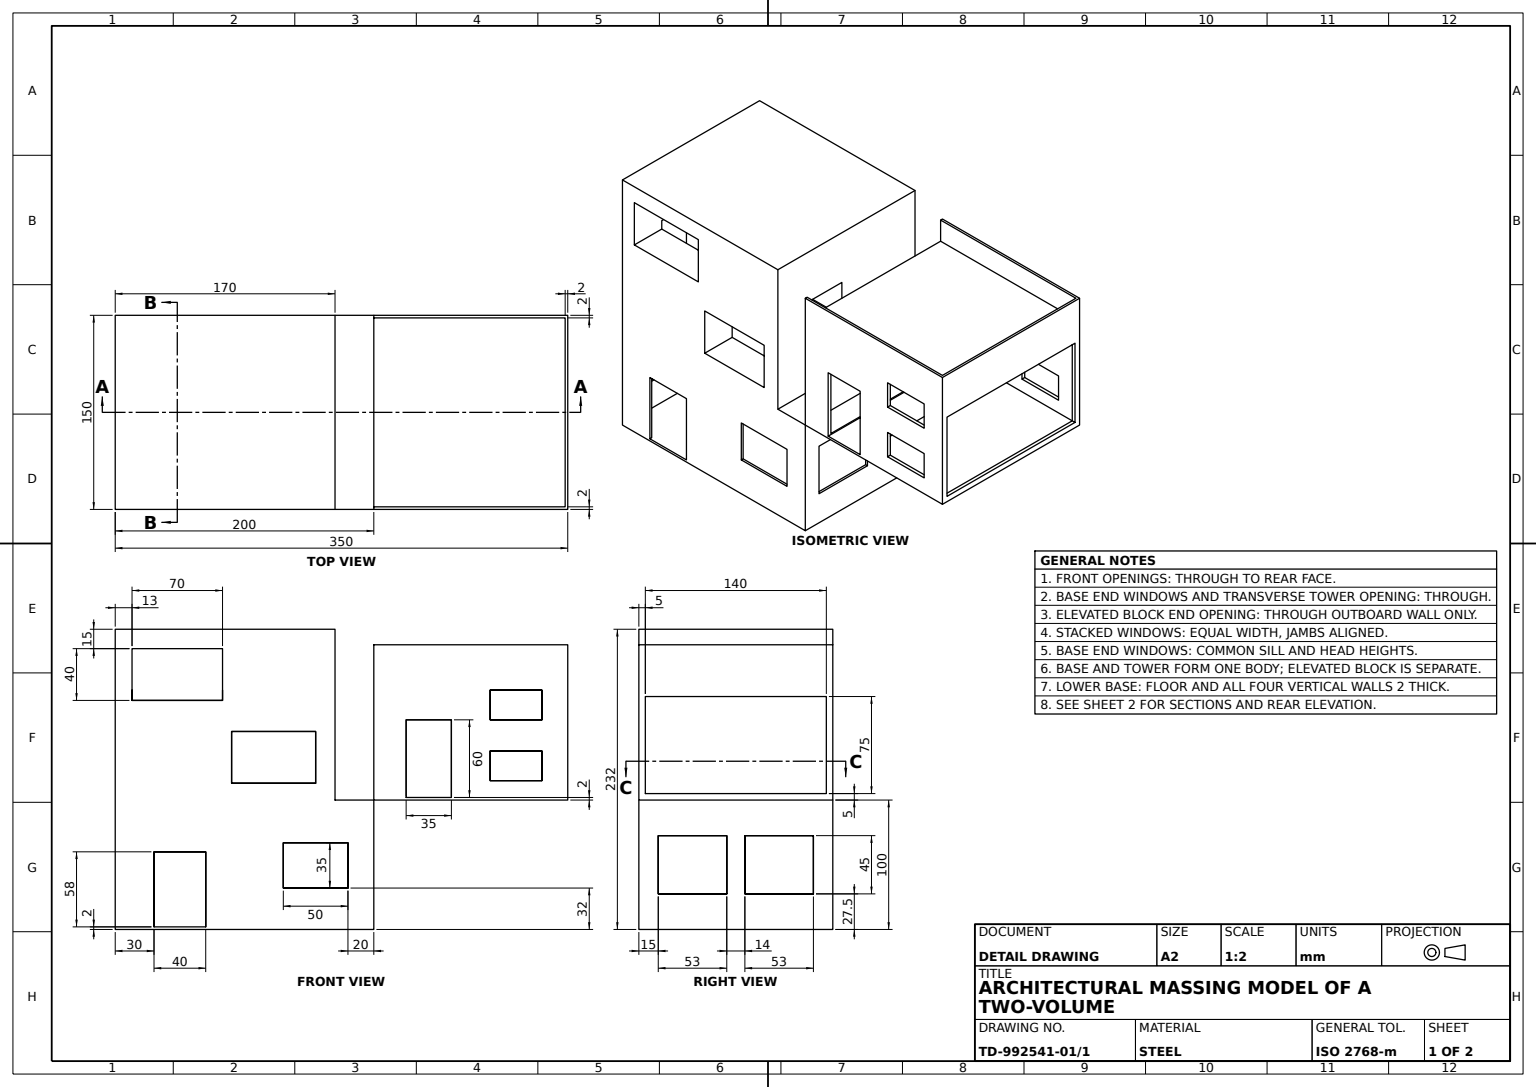
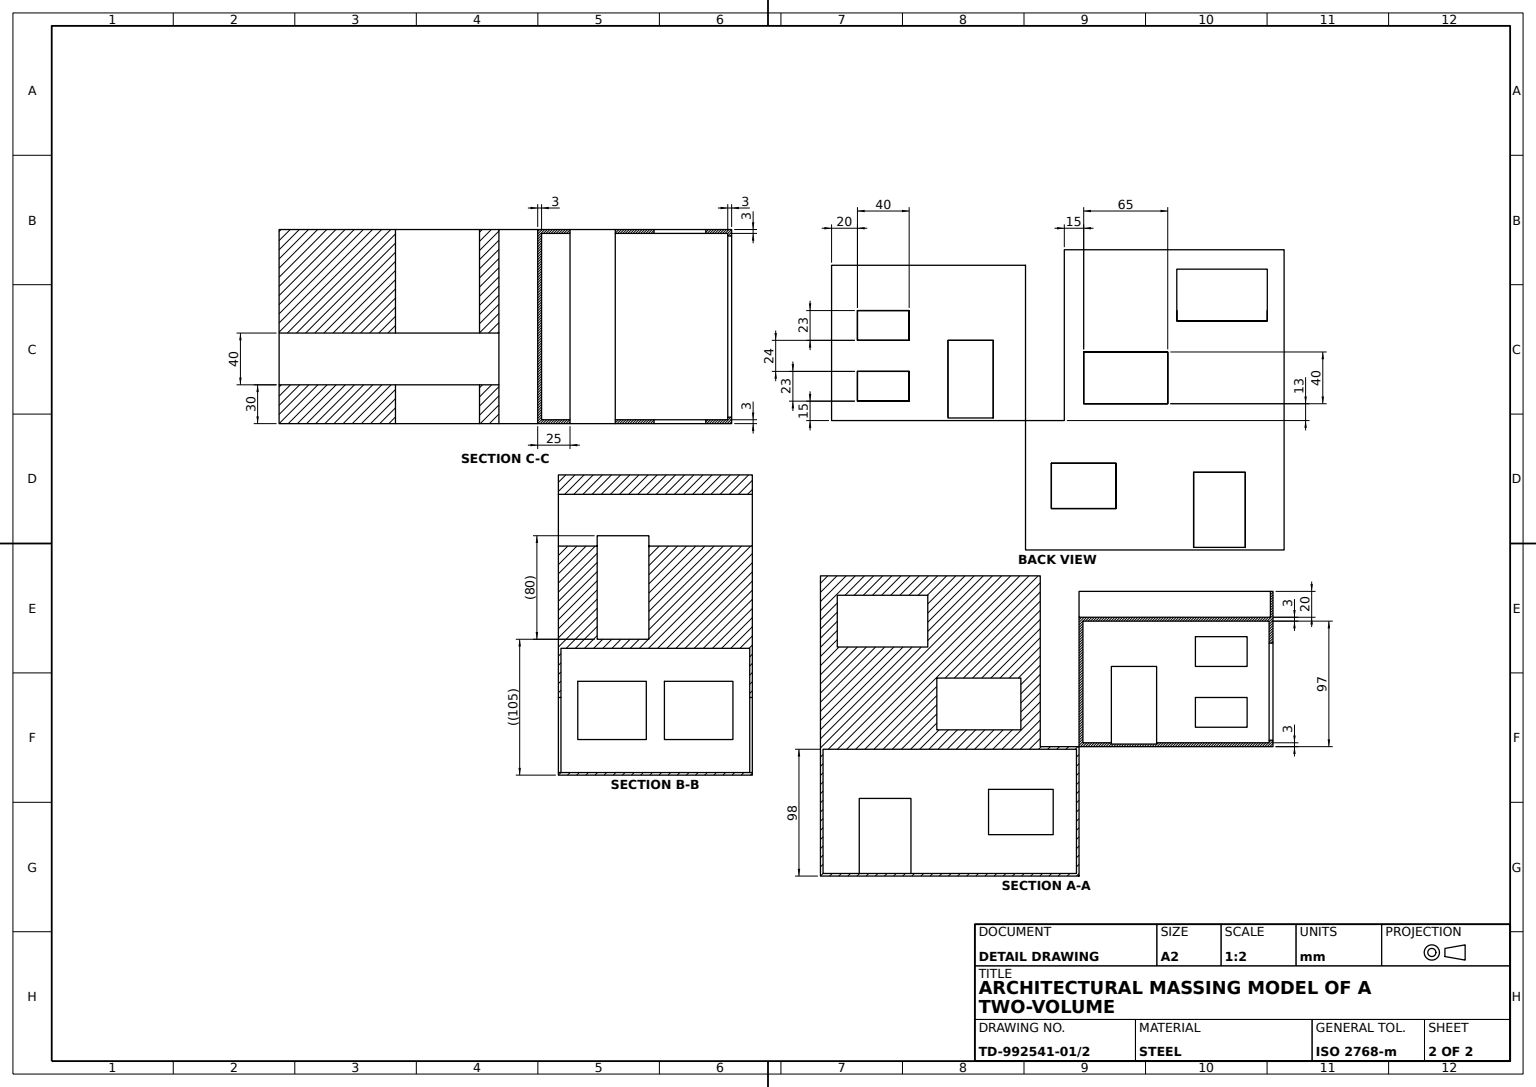
SolidWorks part; units mm, degrees
material "Plain Carbon Steel"
ref_plane "Front Plane" through (0, 0, 0) normal (0, 0, 1) x (1, 0, 0)
ref_plane "Top Plane" through (0, 0, 0) normal (0, 1, 0) x (1, 0, 0)
ref_plane "Right Plane" through (0, 0, 0) normal (1, 0, 0) x (0, 0, -1)
sketch "Base Block Sketch" plane through (0, 0, 0) normal (0, 1, 0) x (1, 0, 0)
  line L1 (0, 0) -> (200, 0)
  line L2 (0, 0) -> (0, 150)
  line L3 (0, 150) -> (200, 150)
  line L4 (200, 0) -> (200, 150)
  dimension "D1" = 200
  dimension "D2" = 150
extrude "Base Block" add sketch "Base Block Sketch" along normal blind 100
sketch "Base Door Opening Sketch" plane through (0, 0, 0) normal (0, 0, 1) x (1, 0, 0)
  line L1 (30, 2) -> (70, 2)
  line L2 (30, 2) -> (30, 60)
  line L3 (30, 60) -> (70, 60)
  line L4 (70, 2) -> (70, 60)
  dimension "D1" = 2
  dimension "D2" = 30
  dimension "D3" = 40
  dimension "D4" = 58
extrude "Base Door Opening" cut sketch "Base Door Opening Sketch" against normal blind 270
sketch "Base Hollow Sketch" plane through (0, 100, 0) normal (0, 1, 0) x (1, 0, 0)
  line L0 (200, 0) -> (200, 150) construction
  line L1 (2, 148) -> (198, 148)
  line L2 (2, 148) -> (2, 2)
  line L3 (2, 2) -> (198, 2)
  line L4 (198, 148) -> (198, 2)
  line L5 (200, 150) -> (0, 150) construction
  line L6 (0, 150) -> (0, 0) construction
  line L7 (0, 0) -> (200, 0) construction
  dimension "D1" = 2
  dimension "D2" = 2
  dimension "D3" = 2
  dimension "D4" = 2
extrude "Base Hollow 2mm Wall" cut sketch "Base Hollow Sketch" against normal blind 98
sketch "Base Floor Slab Sketch" plane through (0, 100, 0) normal (0, 1, 0) x (1, 0, 0)
  line L1 (0, 150) -> (200, 150)
  line L2 (0, 150) -> (0, 0)
  line L3 (0, 0) -> (200, 0)
  line L4 (200, 150) -> (200, 0)
extrude "Base Floor Slab" add sketch "Base Floor Slab Sketch" against normal blind 2
sketch "Base Window Sketch" plane through (0, 0, 0) normal (0, 0, 1) x (1, 0, 0)
  line L1 (130, 32) -> (180, 32)
  line L2 (130, 32) -> (130, 67)
  line L3 (130, 67) -> (180, 67)
  line L4 (180, 32) -> (180, 67)
  dimension "D1" = 32
  dimension "D2" = 35
  dimension "D3" = 50
  dimension "D4" = 20
extrude "Base Window" cut sketch "Base Window Sketch" against normal blind 332
sketch "Base Side Windows Sketch" plane through (200, 0, 0) normal (1, 0, 0) x (0, 0, -1)
  line L0 (0, 0) -> (150, 0) construction
  line L1 (15, 27.5) -> (68, 27.5)
  line L2 (15, 27.5) -> (15, 72.5)
  line L3 (15, 72.5) -> (68, 72.5)
  line L4 (68, 27.5) -> (68, 72.5)
  line L5 (82, 27.5) -> (135, 27.5)
  line L6 (82, 27.5) -> (82, 72.5)
  line L7 (82, 72.5) -> (135, 72.5)
  line L8 (135, 27.5) -> (135, 72.5)
  dimension "D1" = 15
  dimension "D2" = 15
  dimension "D3" = 53
  dimension "D4" = 53
  dimension "D5" = 45
  dimension "D6" = 45
  dimension "D7" = 27.5
  dimension "D8" = 27.5
extrude "Base Side Windows" cut sketch "Base Side Windows Sketch" against normal blind 332
sketch "Side Block Sketch" plane through (0, 100, 0) normal (0, 1, 0) x (1, 0, 0)
  line L1 (200, 0) -> (350, 0)
  line L2 (200, 0) -> (200, 150)
  line L3 (200, 150) -> (350, 150)
  line L4 (350, 0) -> (350, 150)
  dimension "D1" = 150
  dimension "D2" = 150
extrude "Side Block" add sketch "Side Block Sketch" along normal blind 100 separate body
sketch "Side Block Hollow Sketch" plane through (0, 200, 0) normal (0, 1, 0) x (1, 0, 0)
  line L0 (200, 0) -> (350, 0) construction
  line L1 (203, 147) -> (347, 147)
  line L2 (203, 147) -> (203, 3)
  line L3 (203, 3) -> (347, 3)
  line L4 (347, 147) -> (347, 3)
  line L5 (350, 0) -> (350, 150) construction
  line L6 (350, 150) -> (200, 150) construction
  line L7 (200, 150) -> (200, 0) construction
  dimension "D1" = 3
  dimension "D2" = 3
  dimension "D3" = 3
  dimension "D4" = 3
extrude "Side Block Hollow 3mm Wall" cut sketch "Side Block Hollow Sketch" against normal blind 97
sketch "Side Block Floor Slab Sketch" plane through (0, 200, 0) normal (0, 1, 0) x (1, 0, 0)
  line L1 (200, 150) -> (350, 150)
  line L2 (200, 150) -> (200, 0)
  line L3 (200, 0) -> (350, 0)
  line L4 (350, 150) -> (350, 0)
extrude "Side Block Floor Slab" add sketch "Side Block Floor Slab Sketch" against normal blind 3
sketch "Side Block Door Sketch" plane through (0, 0, 0) normal (0, 0, 1) x (1, 0, 0)
  line L1 (225, 102) -> (260, 102)
  line L2 (225, 102) -> (225, 162)
  line L3 (225, 162) -> (260, 162)
  line L4 (260, 102) -> (260, 162)
  dimension "D1" = 2
  dimension "D2" = 25
  dimension "D3" = 35
  dimension "D4" = 60
extrude "Side Block Door Opening" cut sketch "Side Block Door Sketch" against normal blind 213
sketch "Side Block Windows Sketch" plane through (0, 0, 0) normal (0, 0, 1) x (1, 0, 0)
  line L1 (290, 115) -> (330, 115)
  line L2 (290, 115) -> (290, 138)
  line L3 (290, 138) -> (330, 138)
  line L4 (330, 115) -> (330, 138)
  line L5 (290, 162) -> (330, 162)
  line L6 (290, 162) -> (290, 185)
  line L7 (290, 185) -> (330, 185)
  line L8 (330, 162) -> (330, 185)
  dimension "D1" = 15
  dimension "D2" = 15
  dimension "D3" = 23
  dimension "D4" = 23
  dimension "D5" = 40
  dimension "D6" = 40
  dimension "D7" = 20
  dimension "D8" = 20
extrude "Side Block Windows" cut sketch "Side Block Windows Sketch" against normal blind 213
sketch "Side Block Front Opening Sketch" plane through (350, 0, 0) normal (1, 0, 0) x (0, 0, -1)
  line L0 (150, 200) -> (150, 100) construction
  line L1 (5, 105) -> (145, 105)
  line L2 (5, 105) -> (5, 180)
  line L3 (5, 180) -> (145, 180)
  line L4 (145, 105) -> (145, 180)
  dimension "D1" = 5
  dimension "D2" = 75
  dimension "D3" = 5
  dimension "D4" = 140
extrude "Side Block Front Opening" cut sketch "Side Block Front Opening Sketch" against normal blind 113
sketch "Parapet Front Sketch" plane through (0, 0, 0) normal (0, 0, 1) x (1, 0, 0)
  line L1 (200, 200) -> (350, 200)
  line L2 (200, 200) -> (200, 220)
  line L3 (200, 220) -> (350, 220)
  line L4 (350, 200) -> (350, 220)
  dimension "D1" = 20
  dimension "D2" = 150
extrude "Parapet Front" add sketch "Parapet Front Sketch" against normal blind 2
sketch "Parapet Side Sketch" plane through (350, 0, 0) normal (1, 0, 0) x (0, 0, -1)
  line L1 (2, 200) -> (149, 200)
  line L2 (2, 200) -> (2, 220)
  line L3 (2, 220) -> (149, 220)
  line L4 (149, 200) -> (149, 220)
  dimension "D1" = 20
  dimension "D2" = 147
extrude "Parapet Side" add sketch "Parapet Side Sketch" against normal blind 2
sketch "Parapet Back Sketch" plane through (0, 0, -150) normal (0, 0, -1) x (-1, 0, 0)
  line L1 (-350, 220) -> (-200, 220)
  line L2 (-350, 220) -> (-350, 200)
  line L3 (-350, 200) -> (-200, 200)
  line L4 (-200, 220) -> (-200, 200)
extrude "Parapet Back" add sketch "Parapet Back Sketch" against normal blind 2
sketch "Tower Sketch" plane through (0, 100, 0) normal (0, 1, 0) x (1, 0, 0)
  line L0 (0, 0) -> (200, 0) construction
  line L1 (0, 150) -> (170, 150)
  line L2 (0, 150) -> (0, 0)
  line L3 (0, 0) -> (170, 0)
  line L4 (170, 150) -> (170, 0)
  dimension "D1" = 170
extrude "Tower Extension" add sketch "Tower Sketch" along normal blind 132
sketch "Tower Windows Sketch" plane through (0, 0, 0) normal (0, 0, 1) x (1, 0, 0)
  line L0 (0, 232) -> (0, 0) construction
  line L1 (155, 113) -> (90, 113)
  line L2 (155, 113) -> (155, 153)
  line L3 (155, 153) -> (90, 153)
  line L4 (90, 113) -> (90, 153)
  line L5 (13, 217) -> (83, 217)
  line L6 (13, 217) -> (13, 177)
  line L7 (13, 177) -> (83, 177)
  line L8 (83, 217) -> (83, 177)
  line L9 (170, 232) -> (170, 100) construction
  dimension "D1" = 15
  dimension "D2" = 40
  dimension "D3" = 70
  dimension "D4" = 13
  dimension "D5" = 15
  dimension "D6" = 65
  dimension "D7" = 40
  dimension "D8" = 13
extrude "Tower Windows" cut sketch "Tower Windows Sketch" against normal blind 152
sketch "Tower Window Opening Sketch" plane through (170, 0, 0) normal (1, 0, 0) x (0, 0, -1)
  line L0 (5, 105) -> (145, 105) construction
  line L1 (30, 105) -> (70, 105)
  line L2 (30, 105) -> (30, 185)
  line L3 (30, 185) -> (70, 185)
  line L4 (70, 105) -> (70, 185)
  dimension "D1" = 80
  dimension "D2" = 40
  dimension "D3" = 30
extrude "Tower Window Opening" cut sketch "Tower Window Opening Sketch" against normal blind 206
